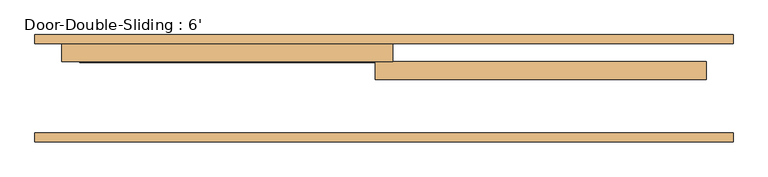
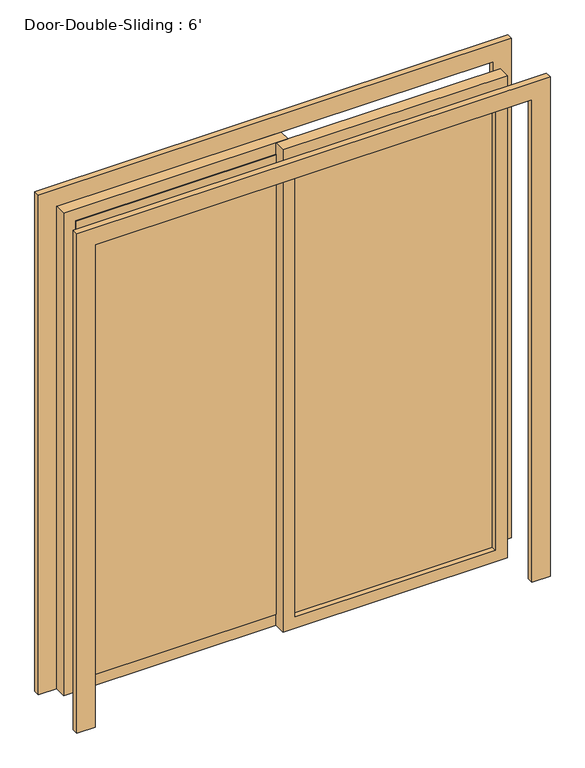
"""IFC4 building model written with IfcOpenShell, lengths in millimetres: door geometry, Door-Double-Sliding : 6'."""

from ifc_helpers import new_model, si_unit, frame, origin, place, context, project, spatial, polyline, outline, extrude, source, transform, mapped, element, save


def door_double_sliding_6_7f701685(model_context):
    return source(origin(), model_context, "Body", "SweptSolid", [
        extrude(outline(polyline([(0.0, 990.6), (2209.8, 990.6), (2209.8, -990.6), (0.0, -990.6), (0.0, -914.4), (2133.6, -914.4), (2133.6, 914.4), (0.0, 914.4), (0.0, 990.6)])), frame((0.0, 254.0, 0.0), z_axis=(0.0, 1.0, 0.0), x_axis=(0.0, 0.0, 1.0)), (0.0, 0.0, 1.0), 25.4),
        extrude(outline(polyline([(0.0, -990.6), (0.0, -914.4), (2133.6, -914.4), (2133.6, 914.4), (0.0, 914.4), (0.0, 990.6), (2209.8, 990.6), (2209.8, -990.6), (0.0, -990.6)])), frame((0.0, -25.4, 0.0), z_axis=(0.0, 1.0, 0.0), x_axis=(0.0, 0.0, 1.0)), (0.0, 0.0, 1.0), 25.4),
        extrude(outline(polyline([(2133.6, 25.4), (2133.6, -914.4), (0.0, -914.4), (0.0, 25.4), (2133.6, 25.4)]), holes=[polyline([(2082.8, -25.4), (50.8, -25.4), (50.8, -863.6), (2082.8, -863.6), (2082.8, -25.4)])]), frame((0.0, 203.2, 0.0), z_axis=(0.0, 1.0, 0.0), x_axis=(0.0, 0.0, 1.0)), (0.0, 0.0, 1.0), 50.8),
        extrude(outline(polyline([(2133.6, -25.4), (0.0, -25.4), (0.0, 914.4), (2133.6, 914.4), (2133.6, -25.4)]), holes=[polyline([(2082.8, 25.4), (2082.8, 863.6), (50.8, 863.6), (50.8, 25.4), (2082.8, 25.4)])]), frame((0.0, 152.4, 0.0), z_axis=(0.0, 1.0, 0.0), x_axis=(0.0, 0.0, 1.0)), (0.0, 0.0, 1.0), 50.8),
        extrude(outline(polyline([(-25.4, 200.025), (-863.6, 200.025), (-863.6, 206.375), (-25.4, 206.375), (-25.4, 200.025)])), frame((0.0, 0.0, 50.8), z_axis=(0.0, 0.0, 1.0), x_axis=(1.0, 0.0, 0.0)), (0.0, 0.0, 1.0), 2032.0),
        extrude(outline(polyline([(25.4, 180.975), (863.6, 180.975), (863.6, 174.625), (25.4, 174.625), (25.4, 180.975)])), frame((0.0, 0.0, 50.8), z_axis=(0.0, 0.0, 1.0), x_axis=(1.0, 0.0, 0.0)), (0.0, 0.0, 1.0), 2032.0),
    ])


if __name__ == "__main__":
    model = new_model("IFC4")
    model_context = context("Model", 3, world=origin())
    ifc_project = project(units=[si_unit("LENGTHUNIT", "METRE", prefix="MILLI")], contexts=[model_context])
    site = spatial("IfcSite", under=ifc_project)
    building = spatial("IfcBuilding", under=site)
    placement = place(None, origin())
    door_double_sliding_6_shape = door_double_sliding_6_7f701685(model_context)
    element("IfcDoor", 1, ObjectType="Door-Double-Sliding : 6'", at=placement, inside=building, context=model_context, shape_type="MappedRepresentation", body=[
        mapped(door_double_sliding_6_shape, transform((0.0, 0.0, 0.0), x_axis=(1.0, 0.0, 0.0), y_axis=(0.0, 1.0, 0.0), z_axis=(0.0, 0.0, 1.0))),
    ])
    save(model, "model.ifc")

# Revit data of these elements
# Type "Door-Double-Sliding : 6'"
#   Type Mark = "17"
#   Construction Type Id = "opn-d45"
#   Assembly Code = "C1020"
#   Analytic Construction = "Wood frame, double glass door "
#   Thickness = 0' - 2"
#   Thermal Resistance (R) = 1.8150 (h·ft²·°F)/BTU
#   Heat Transfer Coefficient (U) = 0.5510 BTU/(h·ft²·°F)
#   Height = 7' - 0"
#   Rail Width = 0' - 2"
#   Stiles = 0' - 2"
#   Trim Projection Ext = 0' - 1"
#   Trim Projection Int = 0' - 1"
#   Trim Width = 0' - 3"
#   Width = 6' - 0"
#   Define Thermal Properties by = 1
#   Glazing = Glass
#   Panel Material = Wood - Birch - Solid Stained Light Low Gloss
#   Trim Material = Paint - Sienna
#   Visual Light Transmittance = 0
#   Solar Heat Gain Coefficient = 0
#   Function = (empty or 0)
#   Wall Closure = (empty or 0)
# Element 1 (IfcDoor, "Door-Double-Sliding : 6'")
#   Materials on its faces: "Paint - Sienna", "Wood - Birch - Solid Stained Light Low Gloss", "Glass"
# Materials
#   "Glass": class "Glass", colour RGB 0 128 192, transparency 0.75, Description = "Soda Lime Glass", Cost = 0
#   "Wood - Birch - Solid Stained Light Low Gloss": class "Wood", colour RGB 210 159 95, transparency 0, Cost = 0
#   "Paint - Sienna": colour RGB 118 70 51, transparency 0, Cost = 0
